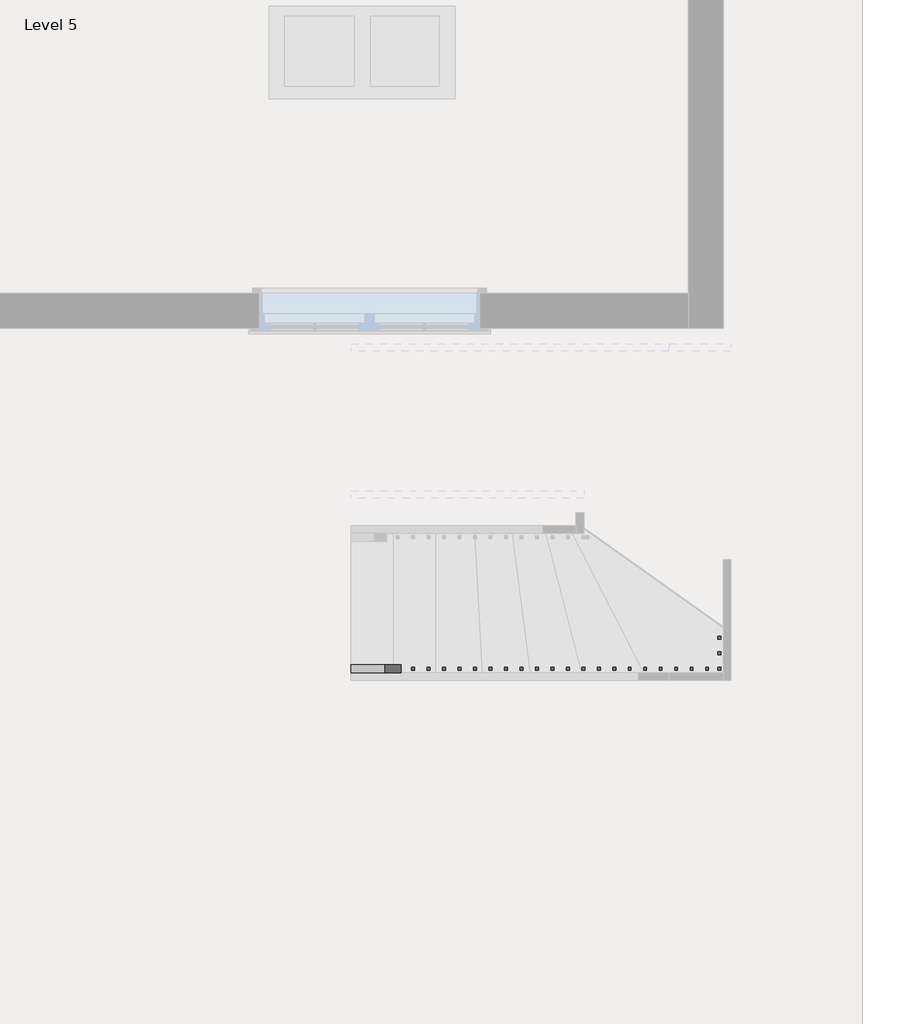
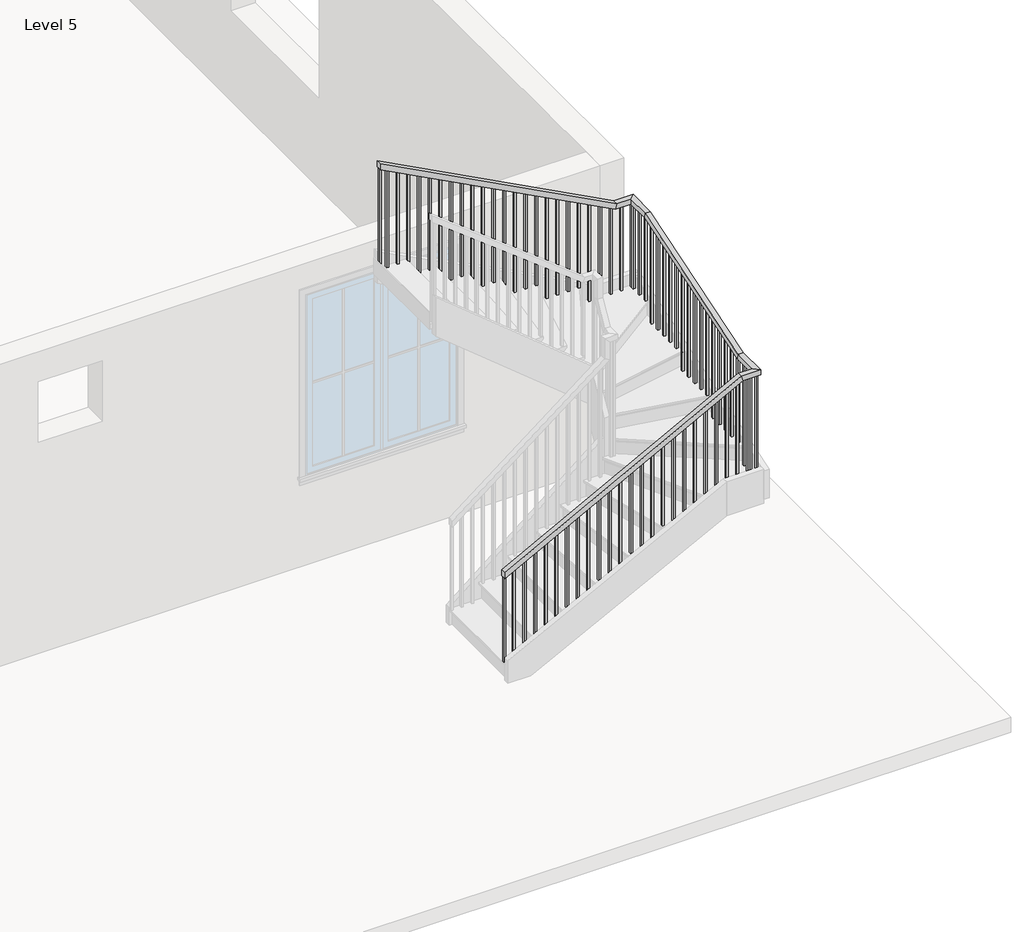
# One storey, part 2 of 3: 1 railing.
"""IFC4 building model written with IfcOpenShell, lengths in millimetres."""

from ifc_helpers import new_model, si_unit, frame, origin, place, context, project, spatial, polyline, outline, extrude, faceted_brep, element, save

model = new_model("IFC4")

# Units and contexts
model_context = context("Model", 3, world=origin())
ifc_project = project(units=[si_unit("LENGTHUNIT", "METRE", prefix="MILLI")], contexts=[model_context])

# Site, building, storey
site = spatial("IfcSite", under=ifc_project)
building = spatial("IfcBuilding", under=site)
storey = spatial("IfcBuildingStorey", under=building, Name="Level 5", Elevation=9601.2)

# Railing
placement = place(None, origin())
element("IfcRailing", 1, ObjectType="Handrail - Rectangular", at=placement, inside=storey, context=model_context, shape_type="SolidModel", body=[
    faceted_brep([(531.7538115, -7514.4090409, 10684.9333333), (531.7538115, -7514.4090409, 10627.4742652), (531.7538115, -7565.2090409, 10627.4742652), (531.7538115, -7565.2090409, 10684.9333333), (2789.4788736, -7514.4090409, 11878.2239201), (2802.0779381, -7514.4090409, 11827.4239201), (2802.0779381, -7565.2090409, 11827.4239201), (2789.4788736, -7565.2090409, 11878.2239201), (2923.0855034, -7269.9465826, 11827.4239201), (2923.0855034, -7277.8971587, 11878.2239201), (2923.0855034, -5744.320923, 12370.3094132), (2923.0855034, -5736.3703469, 12319.5094132), (2973.8855034, -7269.9465826, 11827.4239201), (2973.8855034, -5736.3703469, 12319.5094132), (2973.8855034, -7277.8971587, 11878.2239201), (2973.8855034, -5744.320923, 12370.3094132), (531.7538115, -5507.8090409, 13563.6), (531.7538115, -5457.0090409, 13563.6), (531.7538115, -5457.0090409, 13506.1409318), (531.7538115, -5507.8090409, 13506.1409318), (2776.879809, -5507.8090409, 12319.5094132), (2789.4788736, -5507.8090409, 12370.3094132), (2776.879809, -5457.0090409, 12319.5094132), (2789.4788736, -5457.0090409, 12370.3094132), (2923.0855034, -7514.4090409, 11878.2239201), (2923.0855034, -7514.4090409, 11827.4239201), (2973.8855034, -7565.2090409, 11827.4239201), (2973.8855034, -7565.2090409, 11878.2239201), (2923.0855034, -5507.8090409, 12370.3094132), (2923.0855034, -5507.8090409, 12319.5094132), (2973.8855034, -5457.0090409, 12319.5094132), (2973.8855034, -5457.0090409, 12370.3094132)], [[[0, 1, 2, 3]], [[1, 0, 4, 5]], [[2, 1, 5, 6]], [[3, 2, 6, 7]], [[0, 3, 7, 4]], [[8, 9, 10, 11]], [[12, 8, 11, 13]], [[14, 12, 13, 15]], [[9, 14, 15, 10]], [[16, 17, 18, 19]], [[20, 21, 16, 19]], [[22, 20, 19, 18]], [[23, 22, 18, 17]], [[21, 23, 17, 16]], [[5, 4, 24, 25]], [[6, 5, 25, 26]], [[7, 6, 26, 27]], [[4, 7, 27, 24]], [[25, 24, 9, 8]], [[26, 25, 8, 12]], [[27, 26, 12, 14]], [[24, 27, 14, 9]], [[11, 10, 28, 29]], [[13, 11, 29, 30]], [[15, 13, 30, 31]], [[10, 15, 31, 28]], [[29, 28, 21, 20]], [[30, 29, 20, 22]], [[31, 30, 22, 23]], [[28, 31, 23, 21]]]),
    extrude(outline(polyline([(13458.8597858, 621.2105034), (13468.9284102, 602.1605034), (12479.8666667, 602.1605034), (12479.8666667, 621.2105034), (13458.8597858, 621.2105034)])), frame((0.0, -5491.9340409, 0.0), z_axis=(0.0, 1.0, 0.0), x_axis=(0.0, 0.0, 1.0)), (0.0, 0.0, 1.0), 19.05),
    extrude(outline(polyline([(13405.1604556, 722.8105034), (13415.22908, 703.7605034), (12479.8666667, 703.7605034), (12479.8666667, 722.8105034), (13405.1604556, 722.8105034)])), frame((0.0, -5491.9340409, 0.0), z_axis=(0.0, 1.0, 0.0), x_axis=(0.0, 0.0, 1.0)), (0.0, 0.0, 1.0), 19.05),
    extrude(outline(polyline([(13351.4611254, 824.4105034), (13361.5297498, 805.3605034), (12310.5333333, 805.3605034), (12310.5333333, 824.4105034), (13351.4611254, 824.4105034)])), frame((0.0, -5491.9340409, 0.0), z_axis=(0.0, 1.0, 0.0), x_axis=(0.0, 0.0, 1.0)), (0.0, 0.0, 1.0), 19.05),
    extrude(outline(polyline([(13297.7617952, 926.0105034), (13307.8304196, 906.9605034), (12310.5333333, 906.9605034), (12310.5333333, 926.0105034), (13297.7617952, 926.0105034)])), frame((0.0, -5491.9340409, 0.0), z_axis=(0.0, 1.0, 0.0), x_axis=(0.0, 0.0, 1.0)), (0.0, 0.0, 1.0), 19.05),
    extrude(outline(polyline([(13244.062465, 1027.6105034), (13254.1310894, 1008.5605034), (12310.5333333, 1008.5605034), (12310.5333333, 1027.6105034), (13244.062465, 1027.6105034)])), frame((0.0, -5491.9340409, 0.0), z_axis=(0.0, 1.0, 0.0), x_axis=(0.0, 0.0, 1.0)), (0.0, 0.0, 1.0), 19.05),
    extrude(outline(polyline([(13190.3631348, 1129.2105034), (13200.4317592, 1110.1605034), (12141.2, 1110.1605034), (12141.2, 1129.2105034), (13190.3631348, 1129.2105034)])), frame((0.0, -5491.9340409, 0.0), z_axis=(0.0, 1.0, 0.0), x_axis=(0.0, 0.0, 1.0)), (0.0, 0.0, 1.0), 19.05),
    extrude(outline(polyline([(13136.6638046, 1230.8105034), (13146.732429, 1211.7605034), (12141.2, 1211.7605034), (12141.2, 1230.8105034), (13136.6638046, 1230.8105034)])), frame((0.0, -5491.9340409, 0.0), z_axis=(0.0, 1.0, 0.0), x_axis=(0.0, 0.0, 1.0)), (0.0, 0.0, 1.0), 19.05),
    extrude(outline(polyline([(13082.9644744, 1332.4105034), (13093.0330988, 1313.3605034), (12141.2, 1313.3605034), (12141.2, 1332.4105034), (13082.9644744, 1332.4105034)])), frame((0.0, -5491.9340409, 0.0), z_axis=(0.0, 1.0, 0.0), x_axis=(0.0, 0.0, 1.0)), (0.0, 0.0, 1.0), 19.05),
    extrude(outline(polyline([(13029.2651442, 1434.0105034), (13039.3337686, 1414.9605034), (11971.8666667, 1414.9605034), (11971.8666667, 1434.0105034), (13029.2651442, 1434.0105034)])), frame((0.0, -5491.9340409, 0.0), z_axis=(0.0, 1.0, 0.0), x_axis=(0.0, 0.0, 1.0)), (0.0, 0.0, 1.0), 19.05),
    extrude(outline(polyline([(12975.565814, 1535.6105034), (12985.6344384, 1516.5605034), (11971.8666667, 1516.5605034), (11971.8666667, 1535.6105034), (12975.565814, 1535.6105034)])), frame((0.0, -5491.9340409, 0.0), z_axis=(0.0, 1.0, 0.0), x_axis=(0.0, 0.0, 1.0)), (0.0, 0.0, 1.0), 19.05),
    extrude(outline(polyline([(12921.8664838, 1637.2105034), (12931.9351082, 1618.1605034), (11971.8666667, 1618.1605034), (11971.8666667, 1637.2105034), (12921.8664838, 1637.2105034)])), frame((0.0, -5491.9340409, 0.0), z_axis=(0.0, 1.0, 0.0), x_axis=(0.0, 0.0, 1.0)), (0.0, 0.0, 1.0), 19.05),
    extrude(outline(polyline([(12868.1671536, 1738.8105034), (12878.235778, 1719.7605034), (11802.5333333, 1719.7605034), (11802.5333333, 1738.8105034), (12868.1671536, 1738.8105034)])), frame((0.0, -5491.9340409, 0.0), z_axis=(0.0, 1.0, 0.0), x_axis=(0.0, 0.0, 1.0)), (0.0, 0.0, 1.0), 19.05),
    extrude(outline(polyline([(12814.4678234, 1840.4105034), (12824.5364478, 1821.3605034), (11802.5333333, 1821.3605034), (11802.5333333, 1840.4105034), (12814.4678234, 1840.4105034)])), frame((0.0, -5491.9340409, 0.0), z_axis=(0.0, 1.0, 0.0), x_axis=(0.0, 0.0, 1.0)), (0.0, 0.0, 1.0), 19.05),
    extrude(outline(polyline([(12760.7684932, 1942.0105034), (12770.8371176, 1922.9605034), (11802.5333333, 1922.9605034), (11802.5333333, 1942.0105034), (12760.7684932, 1942.0105034)])), frame((0.0, -5491.9340409, 0.0), z_axis=(0.0, 1.0, 0.0), x_axis=(0.0, 0.0, 1.0)), (0.0, 0.0, 1.0), 19.05),
    extrude(outline(polyline([(12707.069163, 2043.6105034), (12717.1377874, 2024.5605034), (11802.5333333, 2024.5605034), (11802.5333333, 2043.6105034), (12707.069163, 2043.6105034)])), frame((0.0, -5491.9340409, 0.0), z_axis=(0.0, 1.0, 0.0), x_axis=(0.0, 0.0, 1.0)), (0.0, 0.0, 1.0), 19.05),
    extrude(outline(polyline([(12653.3698328, 2145.2105034), (12663.4384572, 2126.1605034), (11633.2, 2126.1605034), (11633.2, 2145.2105034), (12653.3698328, 2145.2105034)])), frame((0.0, -5491.9340409, 0.0), z_axis=(0.0, 1.0, 0.0), x_axis=(0.0, 0.0, 1.0)), (0.0, 0.0, 1.0), 19.05),
    extrude(outline(polyline([(12599.6705026, 2246.8105034), (12609.739127, 2227.7605034), (11633.2, 2227.7605034), (11633.2, 2246.8105034), (12599.6705026, 2246.8105034)])), frame((0.0, -5491.9340409, 0.0), z_axis=(0.0, 1.0, 0.0), x_axis=(0.0, 0.0, 1.0)), (0.0, 0.0, 1.0), 19.05),
    extrude(outline(polyline([(12545.9711724, 2348.4105034), (12556.0397968, 2329.3605034), (11633.2, 2329.3605034), (11633.2, 2348.4105034), (12545.9711724, 2348.4105034)])), frame((0.0, -5491.9340409, 0.0), z_axis=(0.0, 1.0, 0.0), x_axis=(0.0, 0.0, 1.0)), (0.0, 0.0, 1.0), 19.05),
    extrude(outline(polyline([(12492.2718422, 2450.0105034), (12502.3404666, 2430.9605034), (11633.2, 2430.9605034), (11633.2, 2450.0105034), (12492.2718422, 2450.0105034)])), frame((0.0, -5491.9340409, 0.0), z_axis=(0.0, 1.0, 0.0), x_axis=(0.0, 0.0, 1.0)), (0.0, 0.0, 1.0), 19.05),
    extrude(outline(polyline([(12438.572512, 2551.6105034), (12448.6411364, 2532.5605034), (11463.8666667, 2532.5605034), (11463.8666667, 2551.6105034), (12438.572512, 2551.6105034)])), frame((0.0, -5491.9340409, 0.0), z_axis=(0.0, 1.0, 0.0), x_axis=(0.0, 0.0, 1.0)), (0.0, 0.0, 1.0), 19.05),
    extrude(outline(polyline([(12384.8731818, 2653.2105034), (12394.9418062, 2634.1605034), (11463.8666667, 2634.1605034), (11463.8666667, 2653.2105034), (12384.8731818, 2653.2105034)])), frame((0.0, -5491.9340409, 0.0), z_axis=(0.0, 1.0, 0.0), x_axis=(0.0, 0.0, 1.0)), (0.0, 0.0, 1.0), 19.05),
    extrude(outline(polyline([(12331.1738516, 2754.8105034), (12341.242476, 2735.7605034), (11463.8666667, 2735.7605034), (11463.8666667, 2754.8105034), (12331.1738516, 2754.8105034)])), frame((0.0, -5491.9340409, 0.0), z_axis=(0.0, 1.0, 0.0), x_axis=(0.0, 0.0, 1.0)), (0.0, 0.0, 1.0), 19.05),
    extrude(outline(polyline([(2856.4105034, -5472.8840409), (2856.4105034, -5491.9340409), (2837.3605034, -5491.9340409), (2837.3605034, -5472.8840409), (2856.4105034, -5472.8840409)])), frame((0.0, 0.0, 11463.8666667), z_axis=(0.0, 0.0, 1.0), x_axis=(1.0, 0.0, 0.0)), (0.0, 0.0, 1.0), 855.6427466),
    extrude(outline(polyline([(2958.0105034, -5517.3340409), (2938.9605034, -5517.3340409), (2938.9605034, -5498.2840409), (2958.0105034, -5498.2840409), (2958.0105034, -5517.3340409)])), frame((0.0, 0.0, 11463.8666667), z_axis=(0.0, 0.0, 1.0), x_axis=(1.0, 0.0, 0.0)), (0.0, 0.0, 1.0), 855.6427466),
    extrude(outline(polyline([(2958.0105034, -5618.9340409), (2938.9605034, -5618.9340409), (2938.9605034, -5599.8840409), (2958.0105034, -5599.8840409), (2958.0105034, -5618.9340409)])), frame((0.0, 0.0, 11463.8666667), z_axis=(0.0, 0.0, 1.0), x_axis=(1.0, 0.0, 0.0)), (0.0, 0.0, 1.0), 855.6427466),
    extrude(outline(polyline([(2958.0105034, -5720.5340409), (2938.9605034, -5720.5340409), (2938.9605034, -5701.4840409), (2958.0105034, -5701.4840409), (2958.0105034, -5720.5340409)])), frame((0.0, 0.0, 11463.8666667), z_axis=(0.0, 0.0, 1.0), x_axis=(1.0, 0.0, 0.0)), (0.0, 0.0, 1.0), 855.6427466),
    extrude(outline(polyline([(-5822.1340409, 12291.9900316), (-5803.0840409, 12298.1026907), (-5803.0840409, 11294.5333333), (-5822.1340409, 11294.5333333), (-5822.1340409, 12291.9900316)])), frame((2938.9605034, 0.0, 0.0), z_axis=(1.0, 0.0, 0.0), x_axis=(0.0, 1.0, 0.0)), (0.0, 0.0, 1.0), 19.05),
    extrude(outline(polyline([(-5923.7340409, 12259.3891834), (-5904.6840409, 12265.5018425), (-5904.6840409, 11294.5333333), (-5923.7340409, 11294.5333333), (-5923.7340409, 12259.3891834)])), frame((2938.9605034, 0.0, 0.0), z_axis=(1.0, 0.0, 0.0), x_axis=(0.0, 1.0, 0.0)), (0.0, 0.0, 1.0), 19.05),
    extrude(outline(polyline([(-6025.3340409, 12226.7883352), (-6006.2840409, 12232.9009942), (-6006.2840409, 11294.5333333), (-6025.3340409, 11294.5333333), (-6025.3340409, 12226.7883352)])), frame((2938.9605034, 0.0, 0.0), z_axis=(1.0, 0.0, 0.0), x_axis=(0.0, 1.0, 0.0)), (0.0, 0.0, 1.0), 19.05),
    extrude(outline(polyline([(-6126.9340409, 12194.187487), (-6107.8840409, 12200.300146), (-6107.8840409, 11294.5333333), (-6126.9340409, 11294.5333333), (-6126.9340409, 12194.187487)])), frame((2938.9605034, 0.0, 0.0), z_axis=(1.0, 0.0, 0.0), x_axis=(0.0, 1.0, 0.0)), (0.0, 0.0, 1.0), 19.05),
    extrude(outline(polyline([(-6228.5340409, 12161.5866387), (-6209.4840409, 12167.6992978), (-6209.4840409, 11294.5333333), (-6228.5340409, 11294.5333333), (-6228.5340409, 12161.5866387)])), frame((2938.9605034, 0.0, 0.0), z_axis=(1.0, 0.0, 0.0), x_axis=(0.0, 1.0, 0.0)), (0.0, 0.0, 1.0), 19.05),
    extrude(outline(polyline([(-6330.1340409, 12128.9857905), (-6311.0840409, 12135.0984495), (-6311.0840409, 11125.2), (-6330.1340409, 11125.2), (-6330.1340409, 12128.9857905)])), frame((2938.9605034, 0.0, 0.0), z_axis=(1.0, 0.0, 0.0), x_axis=(0.0, 1.0, 0.0)), (0.0, 0.0, 1.0), 19.05),
    extrude(outline(polyline([(-6431.7340409, 12096.3849423), (-6412.6840409, 12102.4976013), (-6412.6840409, 11125.2), (-6431.7340409, 11125.2), (-6431.7340409, 12096.3849423)])), frame((2938.9605034, 0.0, 0.0), z_axis=(1.0, 0.0, 0.0), x_axis=(0.0, 1.0, 0.0)), (0.0, 0.0, 1.0), 19.05),
    extrude(outline(polyline([(-6533.3340409, 12063.784094), (-6514.2840409, 12069.8967531), (-6514.2840409, 11125.2), (-6533.3340409, 11125.2), (-6533.3340409, 12063.784094)])), frame((2938.9605034, 0.0, 0.0), z_axis=(1.0, 0.0, 0.0), x_axis=(0.0, 1.0, 0.0)), (0.0, 0.0, 1.0), 19.05),
    extrude(outline(polyline([(-6634.9340409, 12031.1832458), (-6615.8840409, 12037.2959049), (-6615.8840409, 11125.2), (-6634.9340409, 11125.2), (-6634.9340409, 12031.1832458)])), frame((2938.9605034, 0.0, 0.0), z_axis=(1.0, 0.0, 0.0), x_axis=(0.0, 1.0, 0.0)), (0.0, 0.0, 1.0), 19.05),
    extrude(outline(polyline([(-6736.5340409, 11998.5823976), (-6717.4840409, 12004.6950566), (-6717.4840409, 11125.2), (-6736.5340409, 11125.2), (-6736.5340409, 11998.5823976)])), frame((2938.9605034, 0.0, 0.0), z_axis=(1.0, 0.0, 0.0), x_axis=(0.0, 1.0, 0.0)), (0.0, 0.0, 1.0), 19.05),
    extrude(outline(polyline([(-6838.1340409, 11965.9815494), (-6819.0840409, 11972.0942084), (-6819.0840409, 10955.8666667), (-6838.1340409, 10955.8666667), (-6838.1340409, 11965.9815494)])), frame((2938.9605034, 0.0, 0.0), z_axis=(1.0, 0.0, 0.0), x_axis=(0.0, 1.0, 0.0)), (0.0, 0.0, 1.0), 19.05),
    extrude(outline(polyline([(-6939.7340409, 11933.3807011), (-6920.6840409, 11939.4933602), (-6920.6840409, 10955.8666667), (-6939.7340409, 10955.8666667), (-6939.7340409, 11933.3807011)])), frame((2938.9605034, 0.0, 0.0), z_axis=(1.0, 0.0, 0.0), x_axis=(0.0, 1.0, 0.0)), (0.0, 0.0, 1.0), 19.05),
    extrude(outline(polyline([(-7041.3340409, 11900.7798529), (-7022.2840409, 11906.892512), (-7022.2840409, 10955.8666667), (-7041.3340409, 10955.8666667), (-7041.3340409, 11900.7798529)])), frame((2938.9605034, 0.0, 0.0), z_axis=(1.0, 0.0, 0.0), x_axis=(0.0, 1.0, 0.0)), (0.0, 0.0, 1.0), 19.05),
    extrude(outline(polyline([(-7142.9340409, 11868.1790047), (-7123.8840409, 11874.2916637), (-7123.8840409, 10955.8666667), (-7142.9340409, 10955.8666667), (-7142.9340409, 11868.1790047)])), frame((2938.9605034, 0.0, 0.0), z_axis=(1.0, 0.0, 0.0), x_axis=(0.0, 1.0, 0.0)), (0.0, 0.0, 1.0), 19.05),
    extrude(outline(polyline([(-7244.5340409, 11835.5781565), (-7225.4840409, 11841.6908155), (-7225.4840409, 10955.8666667), (-7244.5340409, 10955.8666667), (-7244.5340409, 11835.5781565)])), frame((2938.9605034, 0.0, 0.0), z_axis=(1.0, 0.0, 0.0), x_axis=(0.0, 1.0, 0.0)), (0.0, 0.0, 1.0), 19.05),
    extrude(outline(polyline([(2958.0105034, -7346.1340409), (2938.9605034, -7346.1340409), (2938.9605034, -7327.0840409), (2958.0105034, -7327.0840409), (2958.0105034, -7346.1340409)])), frame((0.0, 0.0, 10786.5333333), z_axis=(0.0, 0.0, 1.0), x_axis=(1.0, 0.0, 0.0)), (0.0, 0.0, 1.0), 1040.8905868),
    extrude(outline(polyline([(2958.0105034, -7447.7340409), (2938.9605034, -7447.7340409), (2938.9605034, -7428.6840409), (2958.0105034, -7428.6840409), (2958.0105034, -7447.7340409)])), frame((0.0, 0.0, 10786.5333333), z_axis=(0.0, 0.0, 1.0), x_axis=(1.0, 0.0, 0.0)), (0.0, 0.0, 1.0), 1040.8905868),
    extrude(outline(polyline([(2859.0288115, -7549.3340409), (2859.0288115, -7530.2840409), (2878.0788115, -7530.2840409), (2878.0788115, -7549.3340409), (2859.0288115, -7549.3340409)])), frame((0.0, 0.0, 10786.5333333), z_axis=(0.0, 0.0, 1.0), x_axis=(1.0, 0.0, 0.0)), (0.0, 0.0, 1.0), 1040.8905868),
    extrude(outline(polyline([(11813.8938418, 2776.4788115), (11803.8252174, 2757.4288115), (10786.5333333, 2757.4288115), (10786.5333333, 2776.4788115), (11813.8938418, 2776.4788115)])), frame((0.0, -7549.3340409, 0.0), z_axis=(0.0, 1.0, 0.0), x_axis=(0.0, 0.0, 1.0)), (0.0, 0.0, 1.0), 19.05),
    extrude(outline(polyline([(11760.1945116, 2674.8788115), (11750.1258872, 2655.8288115), (10786.5333333, 2655.8288115), (10786.5333333, 2674.8788115), (11760.1945116, 2674.8788115)])), frame((0.0, -7549.3340409, 0.0), z_axis=(0.0, 1.0, 0.0), x_axis=(0.0, 0.0, 1.0)), (0.0, 0.0, 1.0), 19.05),
    extrude(outline(polyline([(11706.4951814, 2573.2788115), (11696.426557, 2554.2288115), (10786.5333333, 2554.2288115), (10786.5333333, 2573.2788115), (11706.4951814, 2573.2788115)])), frame((0.0, -7549.3340409, 0.0), z_axis=(0.0, 1.0, 0.0), x_axis=(0.0, 0.0, 1.0)), (0.0, 0.0, 1.0), 19.05),
    extrude(outline(polyline([(11652.7958512, 2471.6788115), (11642.7272268, 2452.6288115), (10786.5333333, 2452.6288115), (10786.5333333, 2471.6788115), (11652.7958512, 2471.6788115)])), frame((0.0, -7549.3340409, 0.0), z_axis=(0.0, 1.0, 0.0), x_axis=(0.0, 0.0, 1.0)), (0.0, 0.0, 1.0), 19.05),
    extrude(outline(polyline([(11599.096521, 2370.0788115), (11589.0278966, 2351.0288115), (10617.2, 2351.0288115), (10617.2, 2370.0788115), (11599.096521, 2370.0788115)])), frame((0.0, -7549.3340409, 0.0), z_axis=(0.0, 1.0, 0.0), x_axis=(0.0, 0.0, 1.0)), (0.0, 0.0, 1.0), 19.05),
    extrude(outline(polyline([(11545.3971908, 2268.4788115), (11535.3285664, 2249.4288115), (10617.2, 2249.4288115), (10617.2, 2268.4788115), (11545.3971908, 2268.4788115)])), frame((0.0, -7549.3340409, 0.0), z_axis=(0.0, 1.0, 0.0), x_axis=(0.0, 0.0, 1.0)), (0.0, 0.0, 1.0), 19.05),
    extrude(outline(polyline([(11491.6978606, 2166.8788115), (11481.6292362, 2147.8288115), (10617.2, 2147.8288115), (10617.2, 2166.8788115), (11491.6978606, 2166.8788115)])), frame((0.0, -7549.3340409, 0.0), z_axis=(0.0, 1.0, 0.0), x_axis=(0.0, 0.0, 1.0)), (0.0, 0.0, 1.0), 19.05),
    extrude(outline(polyline([(11437.9985304, 2065.2788115), (11427.929906, 2046.2288115), (10617.2, 2046.2288115), (10617.2, 2065.2788115), (11437.9985304, 2065.2788115)])), frame((0.0, -7549.3340409, 0.0), z_axis=(0.0, 1.0, 0.0), x_axis=(0.0, 0.0, 1.0)), (0.0, 0.0, 1.0), 19.05),
    extrude(outline(polyline([(11384.2992002, 1963.6788115), (11374.2305758, 1944.6288115), (10447.8666667, 1944.6288115), (10447.8666667, 1963.6788115), (11384.2992002, 1963.6788115)])), frame((0.0, -7549.3340409, 0.0), z_axis=(0.0, 1.0, 0.0), x_axis=(0.0, 0.0, 1.0)), (0.0, 0.0, 1.0), 19.05),
    extrude(outline(polyline([(11330.59987, 1862.0788115), (11320.5312456, 1843.0288115), (10447.8666667, 1843.0288115), (10447.8666667, 1862.0788115), (11330.59987, 1862.0788115)])), frame((0.0, -7549.3340409, 0.0), z_axis=(0.0, 1.0, 0.0), x_axis=(0.0, 0.0, 1.0)), (0.0, 0.0, 1.0), 19.05),
    extrude(outline(polyline([(11276.9005398, 1760.4788115), (11266.8319154, 1741.4288115), (10447.8666667, 1741.4288115), (10447.8666667, 1760.4788115), (11276.9005398, 1760.4788115)])), frame((0.0, -7549.3340409, 0.0), z_axis=(0.0, 1.0, 0.0), x_axis=(0.0, 0.0, 1.0)), (0.0, 0.0, 1.0), 19.05),
    extrude(outline(polyline([(11223.2012096, 1658.8788115), (11213.1325852, 1639.8288115), (10278.5333333, 1639.8288115), (10278.5333333, 1658.8788115), (11223.2012096, 1658.8788115)])), frame((0.0, -7549.3340409, 0.0), z_axis=(0.0, 1.0, 0.0), x_axis=(0.0, 0.0, 1.0)), (0.0, 0.0, 1.0), 19.05),
    extrude(outline(polyline([(11169.5018794, 1557.2788115), (11159.433255, 1538.2288115), (10278.5333333, 1538.2288115), (10278.5333333, 1557.2788115), (11169.5018794, 1557.2788115)])), frame((0.0, -7549.3340409, 0.0), z_axis=(0.0, 1.0, 0.0), x_axis=(0.0, 0.0, 1.0)), (0.0, 0.0, 1.0), 19.05),
    extrude(outline(polyline([(11115.8025492, 1455.6788115), (11105.7339248, 1436.6288115), (10278.5333333, 1436.6288115), (10278.5333333, 1455.6788115), (11115.8025492, 1455.6788115)])), frame((0.0, -7549.3340409, 0.0), z_axis=(0.0, 1.0, 0.0), x_axis=(0.0, 0.0, 1.0)), (0.0, 0.0, 1.0), 19.05),
    extrude(outline(polyline([(11062.103219, 1354.0788115), (11052.0345946, 1335.0288115), (10109.2, 1335.0288115), (10109.2, 1354.0788115), (11062.103219, 1354.0788115)])), frame((0.0, -7549.3340409, 0.0), z_axis=(0.0, 1.0, 0.0), x_axis=(0.0, 0.0, 1.0)), (0.0, 0.0, 1.0), 19.05),
    extrude(outline(polyline([(11008.4038888, 1252.4788115), (10998.3352644, 1233.4288115), (10109.2, 1233.4288115), (10109.2, 1252.4788115), (11008.4038888, 1252.4788115)])), frame((0.0, -7549.3340409, 0.0), z_axis=(0.0, 1.0, 0.0), x_axis=(0.0, 0.0, 1.0)), (0.0, 0.0, 1.0), 19.05),
    extrude(outline(polyline([(10954.7045586, 1150.8788115), (10944.6359342, 1131.8288115), (10109.2, 1131.8288115), (10109.2, 1150.8788115), (10954.7045586, 1150.8788115)])), frame((0.0, -7549.3340409, 0.0), z_axis=(0.0, 1.0, 0.0), x_axis=(0.0, 0.0, 1.0)), (0.0, 0.0, 1.0), 19.05),
    extrude(outline(polyline([(10901.0052284, 1049.2788115), (10890.936604, 1030.2288115), (9939.8666667, 1030.2288115), (9939.8666667, 1049.2788115), (10901.0052284, 1049.2788115)])), frame((0.0, -7549.3340409, 0.0), z_axis=(0.0, 1.0, 0.0), x_axis=(0.0, 0.0, 1.0)), (0.0, 0.0, 1.0), 19.05),
    extrude(outline(polyline([(10847.3058982, 947.6788115), (10837.2372738, 928.6288115), (9939.8666667, 928.6288115), (9939.8666667, 947.6788115), (10847.3058982, 947.6788115)])), frame((0.0, -7549.3340409, 0.0), z_axis=(0.0, 1.0, 0.0), x_axis=(0.0, 0.0, 1.0)), (0.0, 0.0, 1.0), 19.05),
    extrude(outline(polyline([(10793.606568, 846.0788115), (10783.5379436, 827.0288115), (9939.8666667, 827.0288115), (9939.8666667, 846.0788115), (10793.606568, 846.0788115)])), frame((0.0, -7549.3340409, 0.0), z_axis=(0.0, 1.0, 0.0), x_axis=(0.0, 0.0, 1.0)), (0.0, 0.0, 1.0), 19.05),
    extrude(outline(polyline([(10739.9072378, 744.4788115), (10729.8386134, 725.4288115), (9770.5333333, 725.4288115), (9770.5333333, 744.4788115), (10739.9072378, 744.4788115)])), frame((0.0, -7549.3340409, 0.0), z_axis=(0.0, 1.0, 0.0), x_axis=(0.0, 0.0, 1.0)), (0.0, 0.0, 1.0), 19.05),
    extrude(outline(polyline([(10686.2079076, 642.8788115), (10676.1392831, 623.8288115), (9770.5333333, 623.8288115), (9770.5333333, 642.8788115), (10686.2079076, 642.8788115)])), frame((0.0, -7549.3340409, 0.0), z_axis=(0.0, 1.0, 0.0), x_axis=(0.0, 0.0, 1.0)), (0.0, 0.0, 1.0), 19.05),
    extrude(outline(polyline([(2958.0105034, -5491.9340409), (2938.9605034, -5491.9340409), (2938.9605034, -5472.8840409), (2958.0105034, -5472.8840409), (2958.0105034, -5491.9340409)])), frame((0.0, 0.0, 11463.8666667), z_axis=(0.0, 0.0, 1.0), x_axis=(1.0, 0.0, 0.0)), (0.0, 0.0, 1.0), 855.6427466),
    extrude(outline(polyline([(2938.9605034, -7549.3340409), (2938.9605034, -7530.2840409), (2958.0105034, -7530.2840409), (2958.0105034, -7549.3340409), (2938.9605034, -7549.3340409)])), frame((0.0, 0.0, 10786.5333333), z_axis=(0.0, 0.0, 1.0), x_axis=(1.0, 0.0, 0.0)), (0.0, 0.0, 1.0), 1040.8905868),
    extrude(outline(polyline([(13496.0723074, 550.8038115), (13506.1409318, 531.7538115), (12479.8666667, 531.7538115), (12479.8666667, 550.8038115), (13496.0723074, 550.8038115)])), frame((0.0, -5491.9340409, 0.0), z_axis=(0.0, 1.0, 0.0), x_axis=(0.0, 0.0, 1.0)), (0.0, 0.0, 1.0), 19.05),
    extrude(outline(polyline([(10637.5428896, 550.8038115), (10627.4742652, 531.7538115), (9770.5333333, 531.7538115), (9770.5333333, 550.8038115), (10637.5428896, 550.8038115)])), frame((0.0, -7549.3340409, 0.0), z_axis=(0.0, 1.0, 0.0), x_axis=(0.0, 0.0, 1.0)), (0.0, 0.0, 1.0), 19.05),
])

save(model, "model.ifc")

# Revit data of these elements
# Type "Handrail - Rectangular"
#   Assembly Code = "C2010400"
#   built-in parameter 1008612 = 0.0416667 (stored number, unit not read)
#   built-in parameter 1008611 = 0.0416667 (stored number, unit not read)
#   built-in parameter 1008609 = 0.333333 (stored number, unit not read)
#   built-in parameter 1008604 = 0.166667 (stored number, unit not read)
#   built-in parameter 1008603 = 0.166667 (stored number, unit not read)
#   Railing Height = 3' - 0"
#   built-in parameter 1008630 = 2
#   built-in parameter 1008610 = 2
#   built-in parameter 1008618 = Baluster - Square : 3/4"
# Element 1 (IfcRailing, "Handrail - Rectangular")
#   Phase Created = New Construction
